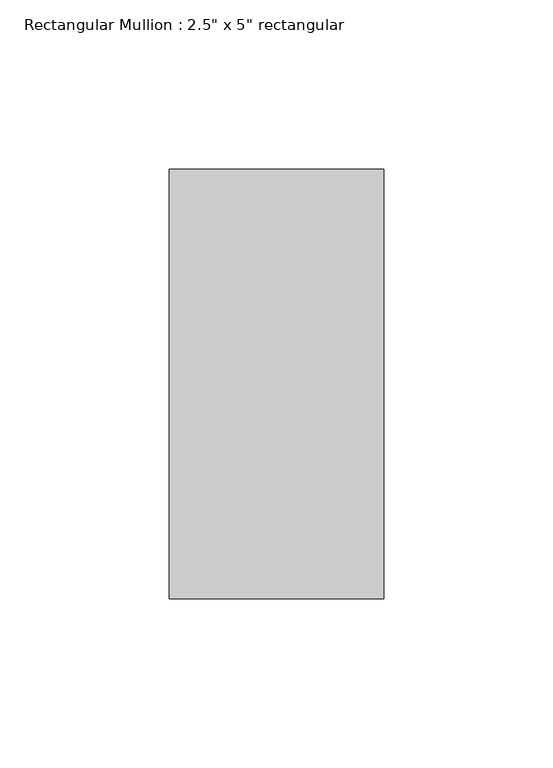
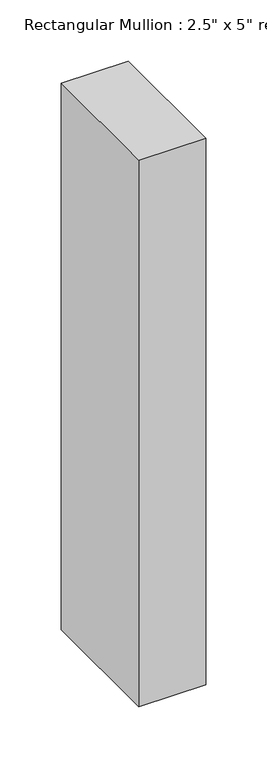
"""IFC4 building model written with IfcOpenShell, lengths in millimetres: member geometry."""

from ifc_helpers import new_model, si_unit, frame, origin, place, context, project, spatial, polyline, outline, extrude, source, transform, mapped, element, save


def member_0a1a1ade(model_context):
    return source(origin(), model_context, "Body", "SweptSolid", [
        extrude(outline(polyline([(31.75, 63.5), (31.75, -63.5), (-31.75, -63.5), (-31.75, 63.5), (31.75, 63.5)])), frame((0.0, 0.0, -546.1), z_axis=(0.0, 0.0, 1.0), x_axis=(1.0, 0.0, 0.0)), (0.0, 0.0, 1.0), 546.1),
    ])


if __name__ == "__main__":
    model = new_model("IFC4")
    model_context = context("Model", 3, world=origin())
    ifc_project = project(units=[si_unit("LENGTHUNIT", "METRE", prefix="MILLI")], contexts=[model_context])
    site = spatial("IfcSite", under=ifc_project)
    building = spatial("IfcBuilding", under=site)
    placement = place(None, origin())
    member_shape = member_0a1a1ade(model_context)
    element("IfcMember", 1, ObjectType="Rectangular Mullion : 2.5\" x 5\" rectangular", at=placement, inside=building, context=model_context, shape_type="MappedRepresentation", body=[
        mapped(member_shape, transform((0.0, 0.0, 0.0), x_axis=(1.0, 0.0, 0.0), y_axis=(0.0, 1.0, 0.0), z_axis=(0.0, 0.0, 1.0))),
    ])
    save(model, "model.ifc")

# Revit data of these elements
# Type "Rectangular Mullion : 2.5\" x 5\" rectangular"
#   built-in parameter 1007304 = 0.416667 (stored number, unit not read)
#   built-in parameter 1007301 = 0.104167 (stored number, unit not read)
#   built-in parameter 1007300 = 0.104167 (stored number, unit not read)
# Element 1 (IfcMember, "Rectangular Mullion : 2.5\" x 5\" rectangular")
#   Materials on its faces: "Aluminum"
# Materials
#   "Aluminum": class "Metal", colour RGB 247 247 247, transparency 0, Description = "Aluminum 6061", Cost = 0
